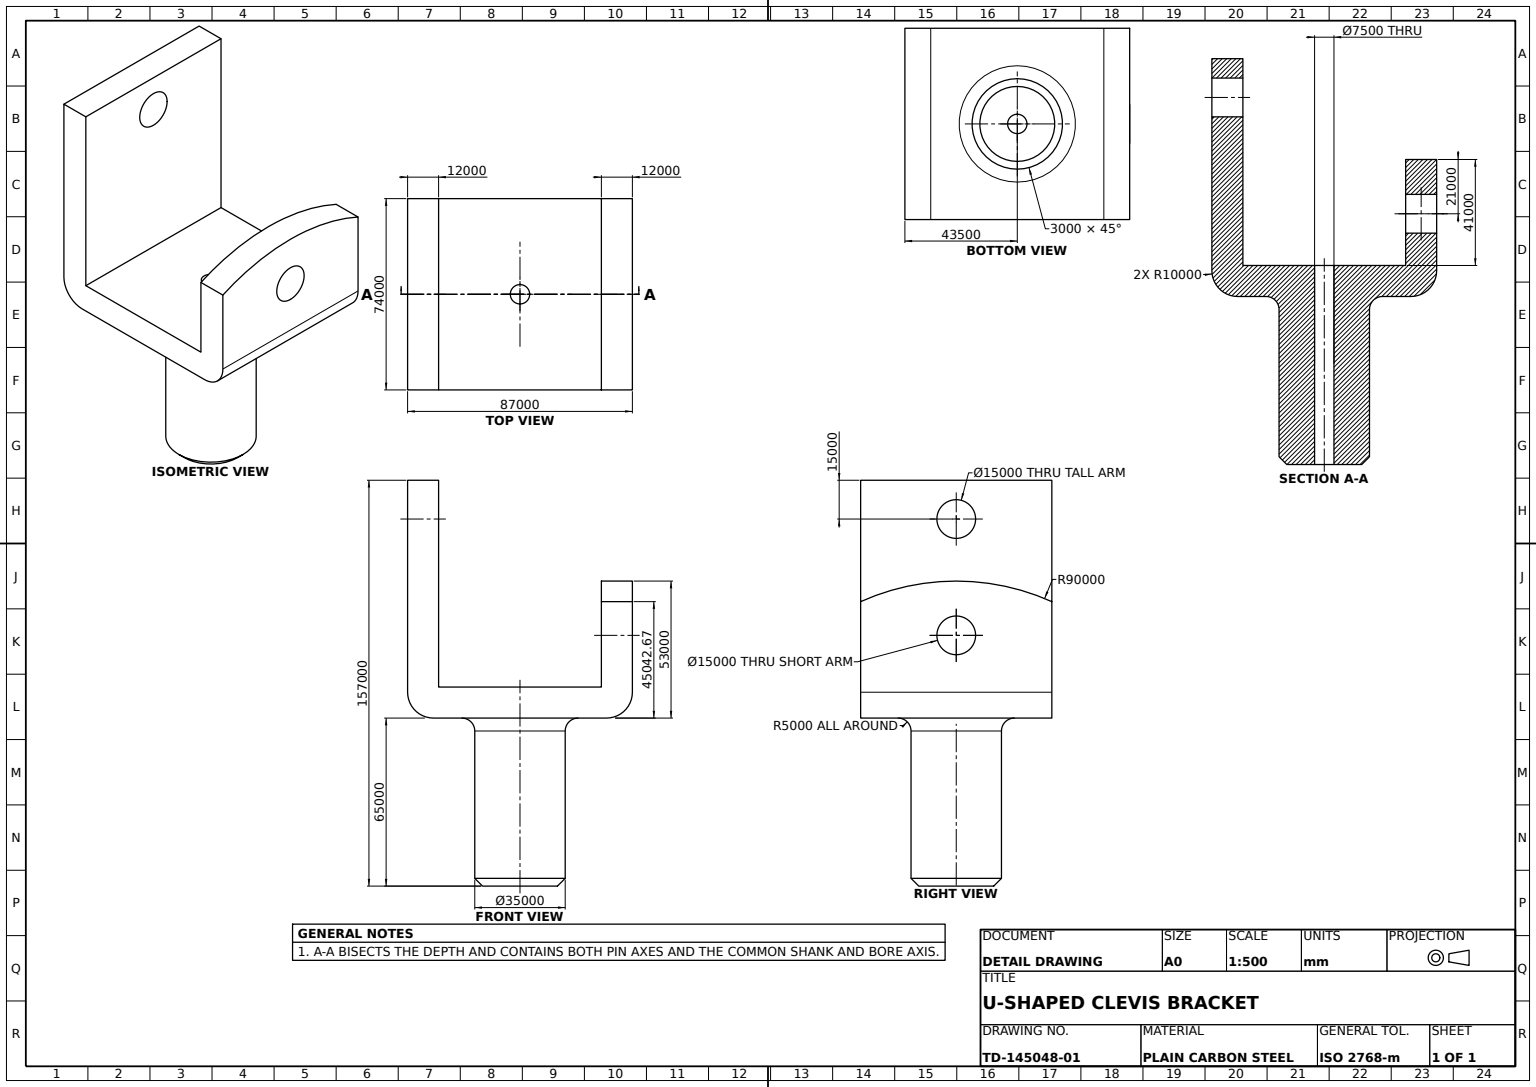
SolidWorks part; units mm, degrees
material "Plain Carbon Steel"
ref_plane "Front Plane" through (0, 0, 0) normal (0, 0, 1) x (1, 0, 0)
ref_plane "Top Plane" through (0, 0, 0) normal (0, 1, 0) x (1, 0, 0)
ref_plane "Right Plane" through (0, 0, 0) normal (1, 0, 0) x (0, 0, -1)
sketch "U Bracket Profile" plane through (0, 0, 0) normal (0, 0, 1) x (1, 0, 0)
  line L1 (-31500, 6000) -> (31500, 6000)
  line L2 (-43500, 6000) -> (-43500, -6000)
  line L3 (-43500, -6000) -> (43500, -6000)
  line L4 (43500, 6000) -> (43500, -6000)
  line L5 (0, 0) -> (43500, -6000) construction
  line L6 (-43500, -6000) -> (0, 0) construction
  line L8 (-43500, 6000) -> (-43500, 86000)
  line L9 (-43500, 86000) -> (-31500, 86000)
  line L10 (-31500, 6000) -> (-31500, 86000)
  line L12 (43500, 6000) -> (43500, 47000)
  line L13 (43500, 47000) -> (31500, 47000)
  line L14 (31500, 6000) -> (31500, 47000)
  point P0 (0, 0)
  dimension "D1" = 12000
  dimension "D2" = 87000
  dimension "D3" = 92000
  dimension "D4" = 12000
  dimension "D5" = 12000
  dimension "D6" = 53000
  dimension "D7" = 41000
  dimension "D8" = 6000
  dimension "D9" = 43500
extrude "U Bracket Body" add sketch "U Bracket Profile" along normal mid plane 74000
fillet "Corner Fillet R10 A" radius 10000 1 edges at (43500, -6000, 0)
fillet "Corner Fillet R10 B" radius 10000 1 edges at (-43500, -6000, 0)
sketch "Short Arm Arc Top Profile" plane through (43500, 0, 0) normal (1, 0, 0) x (0, 0, -1)
  line L4 (-37000, 39042.6718) -> (-37000, 4000)
  line L6 (37000, 4000) -> (37000, 39042.6718)
  line L7 (-37000, 4000) -> (-37000, -6000)
  line L8 (-37000, -6000) -> (37000, -6000)
  line L9 (37000, -6000) -> (37000, 4000)
  arc A0 (37000, 39042.6718) -> (-37000, 39042.6718) centre (0, -43000) ccw
  point P0 (0, 47000)
  dimension "D1" = 53000
  dimension "D2" = 90000
  dimension "D3" = 45042.6718
extrude "Short Arm Arc Top Cut" cut sketch "Short Arm Arc Top Profile" against normal blind 12000 flip side to cut
sketch "Short Arm Pin Hole Sketch" plane through (43500, 0, 0) normal (1, 0, 0) x (0, 0, -1)
  line L0 (0, 47000) -> (0, 26000) construction
  arc A0 (37000, 39042.6718) -> (-37000, 39042.6718) centre (0, -43000) ccw construction
  circle A1 centre (0, 26000) radius 7500
  dimension "D2" = 15000
  dimension "D1" = 21000
extrude "Short Arm Pin Hole" cut sketch "Short Arm Pin Hole Sketch" against normal blind 12000
sketch "Tall Arm Pin Hole Sketch" plane through (-43500, 0, 0) normal (-1, 0, 0) x (0, 0, 1)
  line L0 (0, 86000) -> (0, 71000) construction
  line L1 (37000, 86000) -> (-37000, 86000) construction
  circle A0 centre (0, 71000) radius 7500
  dimension "D2" = 15000
  dimension "D1" = 15000
extrude "Tall Arm Pin Hole" cut sketch "Tall Arm Pin Hole Sketch" against normal blind 12000
sketch "Shank Profile Ø35" plane through (0, -6000, 0) normal (0, -1, 0) x (1, 0, 0)
  circle A0 centre (0, 0) radius 17500
  dimension "D1" = 35000
extrude "Shank Ø35" add sketch "Shank Profile Ø35" along normal blind 65000
fillet "Shank Root Fillet R5" radius 5000 1 edges at (0, -6000, 17500)
chamfer "Shank End Chamfer 3x45" distance 3000 angle 45 1 edges at (0, -71000, -17500)
sketch "Shank Hole Sketch Ø7.5" plane through (0, -71000, 0) normal (0, -1, 0) x (1, 0, 0)
  circle A0 centre (0, 0) radius 3750
  dimension "D1" = 7500
extrude "Shank Hole Ø7.5" cut sketch "Shank Hole Sketch Ø7.5" against normal through all
